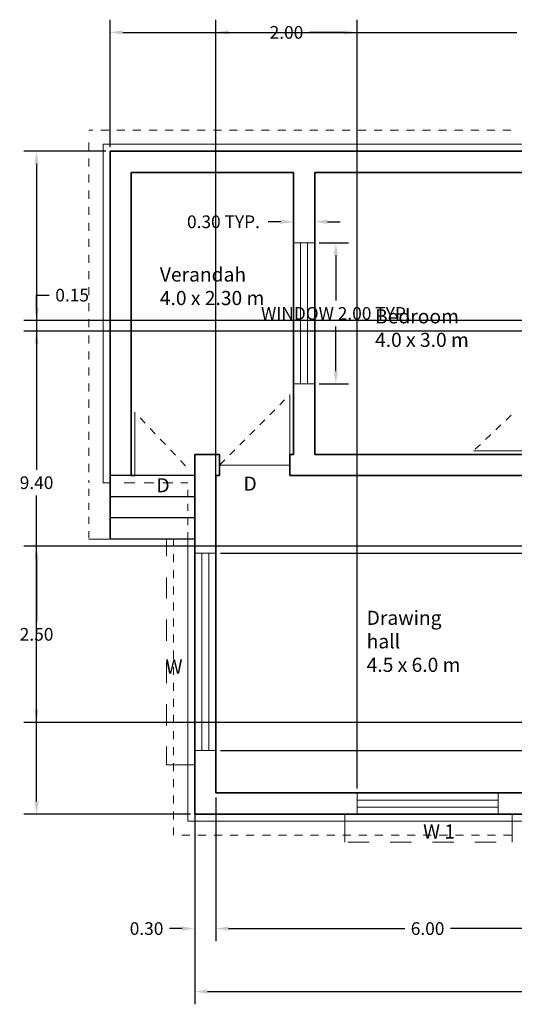
# Model space of a CAD drawing. Units: metres. Extents: x 37.9 to 70.9, y 22.7 to 44.8.
# Tile 1 of 4: x 37.9 to 44.9, y 22.7 to 36.7. Entities that reach past the tile are written whole.
import ezdxf

# ---------------------------------------------------------------- set-up
doc = ezdxf.new("R2010")
doc.units = ezdxf.units.M
doc.header["$LTSCALE"] = 50
doc.header["$MEASUREMENT"] = 0
doc.header["$PDMODE"] = 35
doc.header["$PDSIZE"] = -2
doc.linetypes.add('ACAD_ISO03W100', pattern=[30, 12, -18])
for name, color, linetype, lineweight in [('A-ANNO-DIMS', 2, 'Continuous', 18), ('A-ANNO-TEXT', 7, 'Continuous', 18), ('A-AREA-IDEN', 7, 'Continuous', 18), ('A-DOOR', 4, 'Continuous', 18), ('A-FLOR-PLIN', 7, 'Continuous', 18), ('A-FLOR-STRS', 7, 'Continuous', 25), ('A-GLAZ', 4, 'Continuous', 18), ('A-ROOF-OVHD', 8, 'ACAD_ISO03W100', 13), ('A-WALL', 7, 'Continuous', 35)]:
    doc.layers.add(name, color=color, linetype=linetype, lineweight=lineweight)
doc.styles.get("Standard").update_dxf_attribs({"font": 'arial.ttf'})
doc.dimstyles.get("Standard").update_dxf_attribs({"dimtxt": 0.18, "dimasz": 0.18, "dimexe": 0.18, "dimexo": 0.0625, "dimgap": 0.09, "dimtad": 0, "dimtih": 1, "dimtoh": 1, "dimzin": 0, "dimdsep": 46, "dimtxsty": 'Standard', "dimcen": 0.09, "dimadec": 0, "dimazin": 0, "dimtfac": 1, "dimtofl": 0, "dimtmove": 0, "dimatfit": 3, "dimfxl": 1, "dimtolj": 1, "dimtzin": 0, "dimarcsym": 0})

# ---------------------------------------------------------------- blocks, each defined once
blk = doc.blocks.new('*D6')
at = {"layer": 'A-ANNO-DIMS', "color": 0, "lineweight": -2, "transparency": 16777216}
for p, q in [((40.7, 25.637), (40.7, 23.597)), ((46.7, 25.637), (46.7, 23.597))]:
    blk.add_line(p, q, dxfattribs=at)
at = {"layer": 'A-ANNO-DIMS', "color": 0, "linetype": 'ACAD_ISO03W100', "lineweight": -2, "transparency": 16777216}
for p, q in [((40.88, 23.777), (43.376, 23.777)), ((46.52, 23.777), (44.024, 23.777))]:
    blk.add_line(p, q, dxfattribs=at)
at = {"layer": 'A-ANNO-DIMS', "color": 0, "transparency": 16777216}
for points in [[(40.88, 23.807), (40.88, 23.747), (40.7, 23.777)], [(46.52, 23.807), (46.52, 23.747), (46.7, 23.777)]]:
    blk.add_solid(points, dxfattribs=at)
at = {"layer": 'Defpoints', "color": 0, "transparency": 16777216}
for p in [(40.7, 25.7), (46.7, 25.7), (46.7, 23.777)]:
    blk.add_point(p, dxfattribs=at)
at = {"layer": 'A-ANNO-DIMS', "color": 0, "transparency": 16777216, "insert": (43.7, 23.777), "char_height": 0.18, "attachment_point": 5}
blk.add_mtext('\\A1;6.00', dxfattribs=at)
blk = doc.blocks.new('*D7')
at = {"layer": 'A-ANNO-DIMS', "color": 0, "lineweight": -2, "transparency": 16777216}
for p, q in [((40.4, 25.637), (40.4, 23.597)), ((40.7, 25.637), (40.7, 23.597))]:
    blk.add_line(p, q, dxfattribs=at)
at = {"layer": 'A-ANNO-DIMS', "color": 0, "linetype": 'ACAD_ISO03W100', "lineweight": -2, "transparency": 16777216}
for p, q in [((40.22, 23.777), (40.04, 23.777)), ((40.88, 23.777), (41.06, 23.777))]:
    blk.add_line(p, q, dxfattribs=at)
at = {"layer": 'A-ANNO-DIMS', "color": 0, "transparency": 16777216}
for points in [[(40.22, 23.807), (40.22, 23.747), (40.4, 23.777)], [(40.88, 23.807), (40.88, 23.747), (40.7, 23.777)]]:
    blk.add_solid(points, dxfattribs=at)
at = {"layer": 'Defpoints', "color": 0, "transparency": 16777216}
for p in [(40.4, 25.7), (40.7, 25.7), (40.4, 23.777)]:
    blk.add_point(p, dxfattribs=at)
at = {"layer": 'A-ANNO-DIMS', "color": 0, "transparency": 16777216, "insert": (39.717, 23.777), "char_height": 0.18, "attachment_point": 5}
blk.add_mtext('\\A1;0.30', dxfattribs=at)
blk = doc.blocks.new('*D10')
at = {"layer": 'A-ANNO-DIMS', "color": 0, "lineweight": -2, "transparency": 16777216}
for p, q in [((40.4, 25.337), (40.4, 22.703)), ((51.5, 25.337), (51.5, 22.703))]:
    blk.add_line(p, q, dxfattribs=at)
at = {"layer": 'A-ANNO-DIMS', "color": 0, "linetype": 'ACAD_ISO03W100', "lineweight": -2, "transparency": 16777216}
for p, q in [((40.58, 22.883), (45.565, 22.883)), ((51.32, 22.883), (46.335, 22.883))]:
    blk.add_line(p, q, dxfattribs=at)
at = {"layer": 'A-ANNO-DIMS', "color": 0, "transparency": 16777216}
for points in [[(40.58, 22.913), (40.58, 22.853), (40.4, 22.883)], [(51.32, 22.913), (51.32, 22.853), (51.5, 22.883)]]:
    blk.add_solid(points, dxfattribs=at)
at = {"layer": 'Defpoints', "color": 0, "transparency": 16777216}
for p in [(40.4, 25.4), (51.5, 25.4), (51.5, 22.883)]:
    blk.add_point(p, dxfattribs=at)
at = {"layer": 'A-ANNO-DIMS', "color": 0, "transparency": 16777216, "insert": (45.95, 22.883), "char_height": 0.18, "attachment_point": 5}
blk.add_mtext('\\A1;11.10', dxfattribs=at)
blk = doc.blocks.new('WIN-2000-PLAN')
for p, q in [((0, 0.3), (0, 0)), ((2, 0.3), (2, 0)), ((0, 0.2), (2, 0.2)), ((0, 0.1), (2, 0.1))]:
    blk.add_line(p, q)
blk = doc.blocks.new('*D15')
at = {"layer": 'A-ANNO-DIMS', "color": 0, "lineweight": -2, "transparency": 16777216}
for p, q in [((42.162, 33.5), (42.58, 33.5)), ((42.162, 31.5), (42.58, 31.5))]:
    blk.add_line(p, q, dxfattribs=at)
at = {"layer": 'A-ANNO-DIMS', "color": 0, "linetype": 'ACAD_ISO03W100', "lineweight": -2, "transparency": 16777216}
for p, q in [((42.4, 33.32), (42.4, 32.683)), ((42.4, 31.68), (42.4, 32.317))]:
    blk.add_line(p, q, dxfattribs=at)
at = {"layer": 'A-ANNO-DIMS', "color": 0, "transparency": 16777216}
for points in [[(42.37, 33.32), (42.43, 33.32), (42.4, 33.5)], [(42.37, 31.68), (42.43, 31.68), (42.4, 31.5)]]:
    blk.add_solid(points, dxfattribs=at)
at = {"layer": 'Defpoints', "color": 0, "transparency": 16777216}
for p in [(42.1, 33.5), (42.4, 33.5), (42.1, 31.5)]:
    blk.add_point(p, dxfattribs=at)
at = {"layer": 'A-ANNO-DIMS', "color": 0, "transparency": 16777216, "insert": (42.4, 32.5), "char_height": 0.18, "attachment_point": 5}
blk.add_mtext('\\A1;WINDOW 2.00 TYP.', dxfattribs=at)
blk = doc.blocks.new('*D16')
at = {"layer": 'A-ANNO-DIMS', "color": 0, "lineweight": -2, "transparency": 16777216}
for p, q in [((41.8, 33.563), (41.8, 33.98)), ((42.1, 33.563), (42.1, 33.98))]:
    blk.add_line(p, q, dxfattribs=at)
at = {"layer": 'A-ANNO-DIMS', "color": 0, "linetype": 'ACAD_ISO03W100', "lineweight": -2, "transparency": 16777216}
for p, q in [((41.62, 33.8), (41.44, 33.8)), ((42.28, 33.8), (42.46, 33.8))]:
    blk.add_line(p, q, dxfattribs=at)
at = {"layer": 'A-ANNO-DIMS', "color": 0, "transparency": 16777216}
for points in [[(41.62, 33.83), (41.62, 33.77), (41.8, 33.8)], [(42.28, 33.83), (42.28, 33.77), (42.1, 33.8)]]:
    blk.add_solid(points, dxfattribs=at)
at = {"layer": 'Defpoints', "color": 0, "transparency": 16777216}
for p in [(41.8, 33.8), (41.8, 33.5), (42.1, 33.5)]:
    blk.add_point(p, dxfattribs=at)
at = {"layer": 'A-ANNO-DIMS', "color": 0, "transparency": 16777216, "insert": (40.807, 33.8), "char_height": 0.18, "attachment_point": 5}
blk.add_mtext('\\A1;0.30 TYP.', dxfattribs=at)
blk = doc.blocks.new('*D25')
at = {"layer": 'A-ANNO-DIMS', "color": 0, "linetype": 'ACAD_ISO03W100', "lineweight": -2, "transparency": 16777216}
for p, q in [((38.158, 32.58), (38.158, 32.76)), ((38.158, 32.76), (38.338, 32.76)), ((38.158, 32.07), (38.158, 31.89))]:
    blk.add_line(p, q, dxfattribs=at)
at = {"layer": 'A-ANNO-DIMS', "color": 0, "lineweight": -2, "transparency": 16777216}
for p, q in [((45.338, 32.4), (37.978, 32.4)), ((45.338, 32.25), (37.978, 32.25))]:
    blk.add_line(p, q, dxfattribs=at)
at = {"layer": 'A-ANNO-DIMS', "color": 0, "transparency": 16777216}
for points in [[(38.128, 32.58), (38.188, 32.58), (38.158, 32.4)], [(38.128, 32.07), (38.188, 32.07), (38.158, 32.25)]]:
    blk.add_solid(points, dxfattribs=at)
at = {"layer": 'Defpoints', "color": 0, "transparency": 16777216}
for p in [(38.158, 32.4), (45.4, 32.4), (45.4, 32.25)]:
    blk.add_point(p, dxfattribs=at)
at = {"layer": 'A-ANNO-DIMS', "color": 0, "transparency": 16777216, "insert": (38.662, 32.76), "char_height": 0.18, "attachment_point": 5}
blk.add_mtext('\\A1;0.15', dxfattribs=at)
blk = doc.blocks.new('*D26')
at = {"layer": 'A-ANNO-DIMS', "color": 0, "lineweight": -2, "transparency": 16777216}
for p, q in [((39.2, 34.862), (39.2, 36.666)), ((51.5, 34.862), (51.5, 36.666))]:
    blk.add_line(p, q, dxfattribs=at)
at = {"layer": 'A-ANNO-DIMS', "color": 0, "linetype": 'ACAD_ISO03W100', "lineweight": -2, "transparency": 16777216}
for p, q in [((39.38, 36.486), (44.965, 36.486)), ((51.32, 36.486), (45.735, 36.486))]:
    blk.add_line(p, q, dxfattribs=at)
at = {"layer": 'A-ANNO-DIMS', "color": 0, "transparency": 16777216}
for points in [[(39.38, 36.516), (39.38, 36.456), (39.2, 36.486)], [(51.32, 36.516), (51.32, 36.456), (51.5, 36.486)]]:
    blk.add_solid(points, dxfattribs=at)
at = {"layer": 'Defpoints', "color": 0, "transparency": 16777216}
for p in [(51.5, 36.486), (39.2, 34.8), (51.5, 34.8)]:
    blk.add_point(p, dxfattribs=at)
at = {"layer": 'A-ANNO-DIMS', "color": 0, "transparency": 16777216, "insert": (45.35, 36.486), "char_height": 0.18, "attachment_point": 5}
blk.add_mtext('\\A1;12.30', dxfattribs=at)
blk = doc.blocks.new('*D27')
at = {"layer": 'A-ANNO-DIMS', "color": 0, "lineweight": -2, "transparency": 16777216}
for p, q in [((39.138, 34.8), (37.978, 34.8)), ((40.338, 25.4), (37.978, 25.4))]:
    blk.add_line(p, q, dxfattribs=at)
at = {"layer": 'A-ANNO-DIMS', "color": 0, "linetype": 'ACAD_ISO03W100', "lineweight": -2, "transparency": 16777216}
for p, q in [((38.158, 34.62), (38.158, 30.282)), ((38.158, 25.58), (38.158, 29.918))]:
    blk.add_line(p, q, dxfattribs=at)
at = {"layer": 'A-ANNO-DIMS', "color": 0, "transparency": 16777216}
for points in [[(38.128, 34.62), (38.188, 34.62), (38.158, 34.8)], [(38.128, 25.58), (38.188, 25.58), (38.158, 25.4)]]:
    blk.add_solid(points, dxfattribs=at)
at = {"layer": 'Defpoints', "color": 0, "transparency": 16777216}
for p in [(39.2, 34.8), (38.158, 25.4), (40.4, 25.4)]:
    blk.add_point(p, dxfattribs=at)
at = {"layer": 'A-ANNO-DIMS', "color": 0, "transparency": 16777216, "insert": (38.158, 30.1), "char_height": 0.18, "attachment_point": 5}
blk.add_mtext('\\A1;9.40', dxfattribs=at)
blk = doc.blocks.new('*D28')
at = {"layer": 'A-ANNO-DIMS', "color": 0, "lineweight": -2, "transparency": 16777216}
for p, q in [((40.763, 29.1), (52.823, 29.1)), ((40.763, 26.3), (52.823, 26.3))]:
    blk.add_line(p, q, dxfattribs=at)
at = {"layer": 'A-ANNO-DIMS', "color": 0, "linetype": 'ACAD_ISO03W100', "lineweight": -2, "transparency": 16777216}
for p, q in [((52.643, 28.92), (52.643, 27.882)), ((52.643, 26.48), (52.643, 27.518))]:
    blk.add_line(p, q, dxfattribs=at)
at = {"layer": 'A-ANNO-DIMS', "color": 0, "transparency": 16777216}
for points in [[(52.613, 28.92), (52.673, 28.92), (52.643, 29.1)], [(52.613, 26.48), (52.673, 26.48), (52.643, 26.3)]]:
    blk.add_solid(points, dxfattribs=at)
at = {"layer": 'Defpoints', "color": 0, "transparency": 16777216}
for p in [(40.7, 29.1), (52.643, 29.1), (40.7, 26.3)]:
    blk.add_point(p, dxfattribs=at)
at = {"layer": 'A-ANNO-DIMS', "color": 0, "transparency": 16777216, "insert": (52.643, 27.7), "char_height": 0.18, "attachment_point": 5}
blk.add_mtext('\\A1;2.80', dxfattribs=at)
blk = doc.blocks.new('*D29')
at = {"layer": 'A-ANNO-DIMS', "color": 0, "lineweight": -2, "transparency": 16777216}
for p, q in [((40.7, 25.762), (40.7, 36.666)), ((42.7, 25.762), (42.7, 36.666))]:
    blk.add_line(p, q, dxfattribs=at)
at = {"layer": 'A-ANNO-DIMS', "color": 0, "linetype": 'ACAD_ISO03W100', "lineweight": -2, "transparency": 16777216}
for p, q in [((40.88, 36.486), (41.375, 36.486)), ((42.52, 36.486), (42.025, 36.486))]:
    blk.add_line(p, q, dxfattribs=at)
at = {"layer": 'A-ANNO-DIMS', "color": 0, "transparency": 16777216}
for points in [[(40.88, 36.516), (40.88, 36.456), (40.7, 36.486)], [(42.52, 36.516), (42.52, 36.456), (42.7, 36.486)]]:
    blk.add_solid(points, dxfattribs=at)
at = {"layer": 'Defpoints', "color": 0, "transparency": 16777216}
for p in [(42.7, 36.486), (40.7, 25.7), (42.7, 25.7)]:
    blk.add_point(p, dxfattribs=at)
at = {"layer": 'A-ANNO-DIMS', "color": 0, "transparency": 16777216, "insert": (41.7, 36.486), "char_height": 0.18, "attachment_point": 5}
blk.add_mtext('\\A1;2.00', dxfattribs=at)
blk = doc.blocks.new('*D30')
at = {"layer": 'A-ANNO-DIMS', "color": 0, "lineweight": -2, "transparency": 16777216}
for p, q in [((51.138, 29.2), (37.978, 29.2)), ((51.138, 26.7), (37.978, 26.7))]:
    blk.add_line(p, q, dxfattribs=at)
at = {"layer": 'A-ANNO-DIMS', "color": 0, "linetype": 'ACAD_ISO03W100', "lineweight": -2, "transparency": 16777216}
for p, q in [((38.158, 29.02), (38.158, 28.132)), ((38.158, 26.88), (38.158, 27.768))]:
    blk.add_line(p, q, dxfattribs=at)
at = {"layer": 'A-ANNO-DIMS', "color": 0, "transparency": 16777216}
for points in [[(38.128, 29.02), (38.188, 29.02), (38.158, 29.2)], [(38.128, 26.88), (38.188, 26.88), (38.158, 26.7)]]:
    blk.add_solid(points, dxfattribs=at)
at = {"layer": 'Defpoints', "color": 0, "transparency": 16777216}
for p in [(38.158, 29.2), (51.2, 29.2), (51.2, 26.7)]:
    blk.add_point(p, dxfattribs=at)
at = {"layer": 'A-ANNO-DIMS', "color": 0, "transparency": 16777216, "insert": (38.158, 27.95), "char_height": 0.18, "attachment_point": 5}
blk.add_mtext('\\A1;2.50', dxfattribs=at)

msp = doc.modelspace()

# ---------------------------------------------------------------- linework, layer by layer
at = {"layer": 'A-DOOR'}
for p, q in [((41.75, 30.35), (41.75, 31.35)), ((41.6743, 31.2743), (41.6036, 31.2036)), ((39.55, 30.2), (39.55, 31.1)), ((39.6247, 31.0209), (39.6964, 30.945)), ((41.5328, 31.1328), (41.4621, 31.0621)), ((44.8129, 30.9871), (44.8856, 31.0558)), ((39.7681, 30.8691), (39.8397, 30.7932)), ((41.3914, 30.9914), (41.3207, 30.9207)), ((44.6674, 30.8498), (44.7401, 30.9185)), ((41.25, 30.85), (41.1793, 30.7793)), ((44.5219, 30.7124), (44.5947, 30.7811)), ((39.9114, 30.7173), (39.9831, 30.6415)), ((41.1086, 30.7086), (41.0379, 30.6379)), ((44.3765, 30.575), (44.4492, 30.6437)), ((40.0547, 30.5656), (40.1264, 30.4897)), ((40.9672, 30.5672), (40.8964, 30.4964)), ((45.25, 30.55), (44.35, 30.55)), ((40.198, 30.4138), (40.2697, 30.338)), ((40.8257, 30.4257), (40.75, 30.35)), ((41.75, 30.35), (40.75, 30.35))]:
    msp.add_line(p, q, dxfattribs=at)
at = {"layer": 'A-FLOR-PLIN'}
for p, q in [((39.2, 30.1), (39.0968, 30.1)), ((39.4, 30.1), (39.55, 30.1)), ((39.6811, 30.1), (39.8181, 30.1)), ((39.9455, 30.1), (40.0889, 30.1)), ((40.2034, 30.1), (40.3, 30.1)), ((40.3, 30), (40.3, 29.9)), ((40.3, 29.8), (40.3, 29.7)), ((40.3, 29.6), (40.3, 29.5)), ((40.3, 29.4), (40.3, 29.3))]:
    msp.add_line(p, q, dxfattribs=at)
msp.add_lwpolyline([(39.1, 30.1), (39.1, 34.9), (51.6, 34.9), (51.6, 25.3), (40.3, 25.3), (40.3, 29.3)], dxfattribs=at)
at = {"layer": 'A-FLOR-STRS'}
for p, q in [((40.4, 30.2), (39.2, 30.2)), ((40.4, 29.9), (39.2, 29.9)), ((40.4, 29.6), (39.2, 29.6)), ((40.4, 29.3), (39.2, 29.3))]:
    msp.add_line(p, q, dxfattribs=at)
at = {"layer": 'A-GLAZ'}
for p, q in [((40.4, 29.1), (40.7, 29.1)), ((40.5, 29.1), (40.5, 26.3)), ((40.6, 29.1), (40.6, 26.3)), ((40.4, 26.3), (40.7, 26.3))]:
    msp.add_line(p, q, dxfattribs=at)
at = {"layer": 'A-ROOF-OVHD'}
for p, q in [((38.9, 30.0144), (38.9, 29.9144)), ((38.9, 29.8144), (38.9, 29.7144)), ((38.9, 29.6144), (38.9, 29.5144)), ((38.9, 29.4144), (38.9, 29.3144)), ((39.2, 29.3), (38.9, 29.3)), ((40.4, 29.3), (40, 29.3)), ((40, 29.3), (40, 29.0577)), ((40.4, 29.1), (40.4, 29.3)), ((40, 28.7577), (40, 28.4577)), ((40, 28.1577), (40, 27.8577)), ((40, 27.5577), (40, 27.2577)), ((40, 26.9577), (40, 26.6577)), ((40, 26.3577), (40, 26.1)), ((40, 26.1), (40.4, 26.1)), ((42.5261, 25), (42.5261, 25.4)), ((44.7, 25.4), (44.9, 25.4)), ((44.9, 25.4), (44.9, 25)), ((42.8714, 25), (42.5714, 25)), ((43.4714, 25), (43.1714, 25)), ((44.0714, 25), (43.7714, 25)), ((44.6714, 25), (44.3714, 25))]:
    msp.add_line(p, q, dxfattribs=at)
for points in [[(38.9, 35.1), (38.9536, 35.1)], [(39.0676, 35.1), (39.1816, 35.1)], [(39.2956, 35.1), (39.4096, 35.1)], [(39.5236, 35.1), (39.6376, 35.1)], [(39.7516, 35.1), (39.8656, 35.1)], [(39.9796, 35.1), (40.0936, 35.1)], [(40.2076, 35.1), (40.3216, 35.1)], [(40.4356, 35.1), (40.5496, 35.1)], [(40.6636, 35.1), (40.7776, 35.1)], [(40.8916, 35.1), (41.0056, 35.1)], [(41.1196, 35.1), (41.2336, 35.1)], [(41.3476, 35.1), (41.4616, 35.1)], [(41.5756, 35.1), (41.6896, 35.1)], [(41.8036, 35.1), (41.9176, 35.1)], [(42.0316, 35.1), (42.1456, 35.1)], [(42.2596, 35.1), (42.3736, 35.1)], [(42.4876, 35.1), (42.6016, 35.1)], [(42.7156, 35.1), (42.8296, 35.1)], [(42.9436, 35.1), (43.0576, 35.1)], [(43.1716, 35.1), (43.2856, 35.1)], [(43.3996, 35.1), (43.5137, 35.1)], [(43.6277, 35.1), (43.7417, 35.1)], [(43.8557, 35.1), (43.9697, 35.1)], [(44.0837, 35.1), (44.1977, 35.1)], [(44.3117, 35.1), (44.4257, 35.1)], [(44.5397, 35.1), (44.6537, 35.1)], [(44.7677, 35.1), (44.8817, 35.1)], [(38.9, 34.8116), (38.9, 34.9256)], [(38.9, 34.5836), (38.9, 34.6976)], [(38.9, 34.3556), (38.9, 34.4696)], [(38.9, 34.1276), (38.9, 34.2416)], [(38.9, 33.8996), (38.9, 34.0136)], [(38.9, 33.6716), (38.9, 33.7856)], [(38.9, 33.4436), (38.9, 33.5576)], [(38.9, 33.2156), (38.9, 33.3296)], [(38.9, 32.9876), (38.9, 33.1016)], [(38.9, 32.7596), (38.9, 32.8736)], [(38.9, 32.5316), (38.9, 32.6456)], [(38.9, 32.3036), (38.9, 32.4176)], [(38.9, 32.0756), (38.9, 32.1896)], [(38.9, 31.8476), (38.9, 31.9616)], [(38.9, 31.6196), (38.9, 31.7336)], [(38.9, 31.3916), (38.9, 31.5056)], [(38.9, 31.1636), (38.9, 31.2776)], [(38.9, 30.9356), (38.9, 31.0496)], [(38.9, 30.7076), (38.9, 30.8216)], [(38.9, 30.4796), (38.9, 30.5936)], [(38.9, 30.2516), (38.9, 30.3656)], [(38.9, 30.1), (38.9, 30.1376)], [(40.1, 29.2), (40.1, 29.3)], [(40.1, 28.972), (40.1, 29.086)], [(40.1, 28.744), (40.1, 28.858)], [(40.1, 28.516), (40.1, 28.63)], [(40.1, 28.288), (40.1, 28.402)], [(40.1, 28.06), (40.1, 28.174)], [(40.1, 27.832), (40.1, 27.946)], [(40.1, 27.604), (40.1, 27.718)], [(40.1, 27.376), (40.1, 27.49)], [(40.1, 27.148), (40.1, 27.262)], [(40.1, 26.92), (40.1, 27.034)], [(40.1, 26.692), (40.1, 26.806)], [(40.1, 26.464), (40.1, 26.578)], [(40.1, 26.236), (40.1, 26.35)], [(40.1, 26.008), (40.1, 26.122)], [(40.1, 25.78), (40.1, 25.894)], [(40.1, 25.552), (40.1, 25.666)], [(40.1, 25.324), (40.1, 25.438)], [(40.1, 25.1), (40.1, 25.21)], [(40.332, 25.1), (40.218, 25.1)], [(40.56, 25.1), (40.446, 25.1)], [(40.788, 25.1), (40.674, 25.1)], [(41.0161, 25.1), (40.9021, 25.1)], [(41.2441, 25.1), (41.1301, 25.1)], [(41.4721, 25.1), (41.3581, 25.1)], [(41.7001, 25.1), (41.5861, 25.1)], [(41.9281, 25.1), (41.8141, 25.1)], [(42.1561, 25.1), (42.0421, 25.1)], [(42.3841, 25.1), (42.2701, 25.1)], [(42.6121, 25.1), (42.4981, 25.1)], [(42.8401, 25.1), (42.7261, 25.1)], [(43.0681, 25.1), (42.9541, 25.1)], [(43.2961, 25.1), (43.1821, 25.1)], [(43.5241, 25.1), (43.4101, 25.1)], [(43.7521, 25.1), (43.6381, 25.1)], [(43.9801, 25.1), (43.8661, 25.1)], [(44.2081, 25.1), (44.0941, 25.1)], [(44.4361, 25.1), (44.3221, 25.1)], [(44.6641, 25.1), (44.5501, 25.1)], [(44.8921, 25.1), (44.7781, 25.1)]]:
    msp.add_lwpolyline(points, dxfattribs=at)
at = {"layer": 'A-WALL'}
for p, q in [((39.2, 29.3), (39.2, 34.8)), ((39.2, 34.8), (51.5, 34.8)), ((39.5, 34.5), (41.8, 34.5)), ((39.5, 30.2), (39.5, 34.5)), ((41.8, 34.5), (41.8, 30.5)), ((42.1, 34.5), (42.1, 30.5)), ((42.1, 34.5), (47.9, 34.5)), ((40.4, 30.5), (40.4, 25.4)), ((40.75, 30.5), (40.4, 30.5)), ((40.75, 30.2), (40.75, 30.5)), ((41.8, 30.5), (41.75, 30.5)), ((41.75, 30.5), (41.75, 30.2)), ((45.7966, 30.5), (42.1, 30.5)), ((39.5, 30.2), (39.55, 30.2)), ((40.7, 30.2), (40.7, 25.7)), ((40.75, 30.2), (40.7, 30.2)), ((45.7966, 30.2), (41.75, 30.2)), ((46.7, 25.7), (40.7, 25.7)), ((51.5, 25.4), (40.4, 25.4))]:
    msp.add_line(p, q, dxfattribs=at)

# ---------------------------------------------------------------- block references
at = {"layer": 'A-GLAZ', "rotation": 89.99999999999987}
msp.add_blockref('WIN-2000-PLAN', (42.1, 31.5), dxfattribs=at)
at = {"layer": 'A-GLAZ'}
msp.add_blockref('WIN-2000-PLAN', (42.7, 25.4), dxfattribs=at)

# ---------------------------------------------------------------- texts
at = {"layer": 'A-ANNO-TEXT', "char_height": 0.2, "attachment_point": 1}
for s, insert in [('D', (39.857, 30.1638)), ('D', (41.0916, 30.1865)), ('W', (39.9872, 27.5934)), ('W 1', (43.6368, 25.2541))]:
    msp.add_mtext_dynamic_manual_height_columns(s, width=0.601082, gutter_width=1, heights=[0], dxfattribs=dict(at, insert=insert))
at = {"layer": 'A-AREA-IDEN', "char_height": 0.2, "attachment_point": 1}
for s, insert in [('Verandah\\P4.0 x 2.30 m', (39.9054, 33.1523)), ('Bedroom\\P4.0 x 3.0 m', (42.9552, 32.5588)), ('Drawing hall\\P4.5 x 6.0 m', (42.8367, 28.2839))]:
    msp.add_mtext_dynamic_manual_height_columns(s, width=1.544693, gutter_width=1, heights=[0], dxfattribs=dict(at, insert=insert))

# ---------------------------------------------------------------- dimensions: what is measured, and where the dimension line sits
at = {"layer": 'A-ANNO-DIMS'}
for base, p1, p2, override, picture, middle in [((51.5, 36.4858), (39.2, 34.8), (51.5, 34.8), {"dimdec": 2, "dimlfac": 1, "dimrnd": 0, "dimzin": 0, "dimdsep": 46, "dimlunit": 2}, '*D26', (45.35, 36.4858)), ((42.7, 36.4858), (40.7, 25.7), (42.7, 25.7), {"dimdec": 2, "dimlfac": 1, "dimrnd": 0, "dimzin": 0, "dimdsep": 46, "dimlunit": 2}, '*D29', (41.7, 36.4858)), ((40.4, 23.7769), (40.7, 25.7), (40.4, 25.7), {"dimclrd": 0, "dimclre": 0, "dimclrt": 0}, '*D7', (39.7165, 23.7769)), ((46.7, 23.7769), (40.7, 25.7), (46.7, 25.7), {"dimclrd": 0, "dimclre": 0, "dimclrt": 0}, '*D6', (43.7, 23.7769)), ((51.5, 22.8831), (40.4, 25.4), (51.5, 25.4), {"dimclrd": 0, "dimclre": 0, "dimclrt": 0}, '*D10', (45.95, 22.8831))]:
    dim = msp.add_linear_dim(base=base, p1=p1, p2=p2, dimstyle='Standard', override=override, dxfattribs=at)
    dim.commit()
    dim.dimension.update_dxf_attribs({"geometry": picture, "text_midpoint": middle})
for base, p1, p2, picture, middle in [((38.1575, 25.4), (39.2, 34.8), (40.4, 25.4), '*D27', (38.1575, 30.1)), ((38.1575, 32.4), (45.4, 32.25), (45.4, 32.4), '*D25', (38.662, 32.76)), ((38.1575, 29.2), (51.2, 26.7), (51.2, 29.2), '*D30', (38.1575, 27.95)), ((52.6425, 29.1), (40.7, 26.3), (40.7, 29.1), '*D28', (52.6425, 27.7))]:
    dim = msp.add_linear_dim(base=base, p1=p1, p2=p2, angle=90, dimstyle='Standard', override={"dimdec": 2, "dimlfac": 1, "dimrnd": 0, "dimzin": 0, "dimdsep": 46, "dimlunit": 2}, dxfattribs=at)
    dim.commit()
    dim.dimension.update_dxf_attribs({"geometry": picture, "text_midpoint": middle})
for base, p1, p2, angle, text, picture, middle in [((41.8, 33.8), (42.1, 33.5), (41.8, 33.5), 180, '<> TYP.', '*D16', (40.8071, 33.8)), ((42.4, 33.5), (42.1, 31.5), (42.1, 33.5), 90, 'WINDOW <> TYP.', '*D15', (42.4, 32.5))]:
    dim = msp.add_linear_dim(base=base, p1=p1, p2=p2, angle=angle, text=text, dimstyle='Standard', override={"dimdec": 2, "dimlfac": 1, "dimrnd": 0, "dimzin": 0, "dimdsep": 46, "dimlunit": 2}, dxfattribs=at)
    dim.commit()
    dim.dimension.update_dxf_attribs({"geometry": picture, "text_midpoint": middle})

doc.saveas('drawing.dxf')
